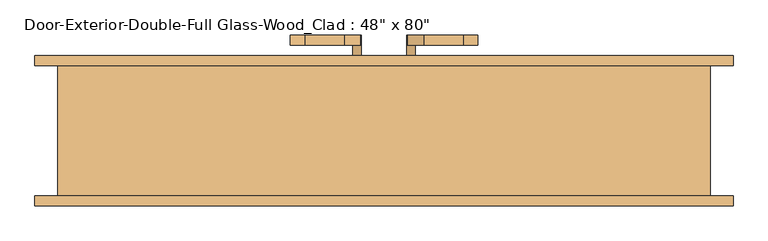
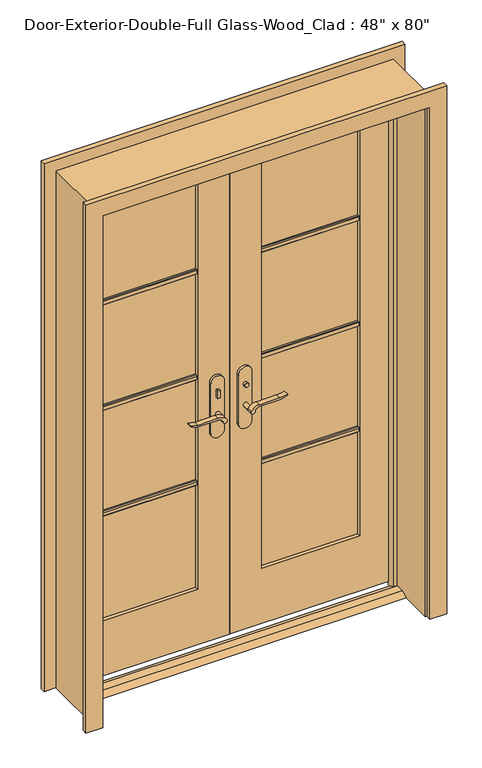
"""IFC4 building model written with IfcOpenShell, lengths in millimetres: door geometry."""

from ifc_helpers import new_model, si_unit, point, frame, frame_2d, origin, place, context, project, spatial, polyline, circle_curve, trimmed, segment, composite_curve, outline, extrude, faceted_brep, source, transform, mapped, element, save


def door_ae07d0c6(model_context):
    return source(origin(), model_context, "Body", "SolidModel", [
        extrude(outline(polyline([(19.05, 12.7), (53.975, 12.7), (79.375, 0.0), (-6.35, 0.0), (19.05, 12.7)])), frame((-609.6, 0.0, 0.0), z_axis=(1.0, 0.0, 0.0), x_axis=(0.0, 1.0, 0.0)), (0.0, 0.0, 1.0), 1219.2),
        extrude(outline(polyline([(-47.4019111, 68.9), (-57.4019111, 68.9), (-57.4019111, 78.9), (-47.4019111, 78.9), (-47.4019111, 68.9)])), frame((0.0, 0.0, 981.9), z_axis=(0.0, 0.0, 1.0), x_axis=(1.0, 0.0, 0.0)), (0.0, 0.0, 1.0), 30.0),
        extrude(outline(composite_curve([segment(trimmed(circle_curve(frame_2d((996.9, -52.4019111)), 8.0), [point((996.9, -60.4019111))], [point((996.9, -44.4019111))], False, "CARTESIAN"), True, "CONTINUOUS"), segment(trimmed(circle_curve(frame_2d((996.9, -52.4019111)), 8.0), [point((996.9, -44.4019111))], [point((996.9, -60.4019111))], False, "CARTESIAN"), True, "CONTINUOUS")], self_intersect=False)), frame((0.0, 133.825, 0.0), z_axis=(0.0, 1.0, 0.0), x_axis=(0.0, 0.0, 1.0)), (0.0, 0.0, 1.0), 10.0),
        extrude(outline(composite_curve([segment(trimmed(circle_curve(frame_2d((897.1555521, -76.0694241)), 37.2832219), [point((919.0523287, -45.8937749))], [point((934.4, -77.7693445))], False, "CARTESIAN"), True, "CONTINUOUS"), segment(polyline([(934.4, -77.7693445), (934.4, -154.045502)]), True, "CONTINUOUS"), segment(trimmed(circle_curve(frame_2d((1017.6850638, -153.9791202)), 83.2850902), [point((934.4, -154.045502))], [point((939.4, -182.4019111))], True, "CARTESIAN"), True, "CONTINUOUS"), segment(polyline([(939.4, -182.4019111), (936.6135558, -182.4019111)]), True, "CONTINUOUS"), segment(trimmed(circle_curve(frame_2d((986.6709207, -150.4622499)), 59.3791355), [point((936.6135558, -182.4019111))], [point((927.4, -154.045502))], False, "CARTESIAN"), True, "CONTINUOUS"), segment(polyline([(927.4, -154.045502), (927.4, -77.7881013)]), True, "CONTINUOUS"), segment(trimmed(circle_curve(frame_2d((909.2738613, -77.7881013)), 18.1261387), [point((927.4, -77.7881013))], [point((914.4, -60.4019111))], True, "CARTESIAN"), True, "CONTINUOUS"), segment(trimmed(circle_curve(frame_2d((914.4, -52.4019111)), 8.0), [point((914.4, -60.4019111))], [point((919.0523287, -45.8937749))], False, "CARTESIAN"), True, "CONTINUOUS")], self_intersect=False)), frame((0.0, 28.9, 0.0), z_axis=(0.0, 1.0, 0.0), x_axis=(0.0, 0.0, 1.0)), (0.0, 0.0, 1.0), 20.0),
        extrude(outline(composite_curve([segment(trimmed(circle_curve(frame_2d((914.4, -52.4019111)), 8.0), [point((914.3999903, -60.4019111))], [point((919.0523287, -45.8937749))], False, "CARTESIAN"), True, "CONTINUOUS"), segment(trimmed(circle_curve(frame_2d((897.1555521, -76.0694241)), 37.2832219), [point((919.0523287, -45.8937749))], [point((934.4, -77.7693445))], False, "CARTESIAN"), True, "CONTINUOUS"), segment(polyline([(934.4, -77.7693445), (934.4, -154.045502)]), True, "CONTINUOUS"), segment(trimmed(circle_curve(frame_2d((1017.6850638, -153.9791202)), 83.2850902), [point((934.4, -154.045502))], [point((939.4, -182.4019111))], True, "CARTESIAN"), True, "CONTINUOUS"), segment(polyline([(939.4, -182.4019111), (936.6135558, -182.4019111)]), True, "CONTINUOUS"), segment(trimmed(circle_curve(frame_2d((986.6709207, -150.4622499)), 59.3791355), [point((936.6135558, -182.4019111))], [point((927.4, -154.045502))], False, "CARTESIAN"), True, "CONTINUOUS"), segment(polyline([(927.4, -154.045502), (927.4, -77.788099)]), True, "CONTINUOUS"), segment(trimmed(circle_curve(frame_2d((909.2738682, -77.788099)), 18.1261318), [point((927.4, -77.788099))], [point((914.3999903, -60.4019111))], True, "CARTESIAN"), True, "CONTINUOUS")], self_intersect=False)), frame((0.0, 163.825, 0.0), z_axis=(0.0, 1.0, 0.0), x_axis=(0.0, 0.0, 1.0)), (0.0, 0.0, 1.0), 20.0),
        extrude(outline(composite_curve([segment(trimmed(circle_curve(frame_2d((914.4, -52.4019111)), 8.0), [point((914.4, -60.4019111))], [point((914.4, -44.4019111))], False, "CARTESIAN"), True, "CONTINUOUS"), segment(trimmed(circle_curve(frame_2d((914.4, -52.4019111)), 8.0), [point((914.4, -44.4019111))], [point((914.4, -60.4019111))], False, "CARTESIAN"), True, "CONTINUOUS")], self_intersect=False)), frame((0.0, 48.9, 0.0), z_axis=(0.0, 1.0, 0.0), x_axis=(0.0, 0.0, 1.0)), (0.0, 0.0, 1.0), 30.0),
        extrude(outline(composite_curve([segment(trimmed(circle_curve(frame_2d((914.4, -52.4019111)), 8.0), [point((914.4, -60.4019111))], [point((914.4, -44.4019111))], False, "CARTESIAN"), True, "CONTINUOUS"), segment(trimmed(circle_curve(frame_2d((914.4, -52.4019111)), 8.0), [point((914.4, -44.4019111))], [point((914.4, -60.4019111))], False, "CARTESIAN"), True, "CONTINUOUS")], self_intersect=False)), frame((0.0, 133.825, 0.0), z_axis=(0.0, 1.0, 0.0), x_axis=(0.0, 0.0, 1.0)), (0.0, 0.0, 1.0), 30.0),
        extrude(outline(composite_curve([segment(polyline([(844.4, -27.4019111), (1039.4, -27.4019111)]), True, "CONTINUOUS"), segment(trimmed(circle_curve(frame_2d((1039.4, -52.4019111)), 25.0), [point((1039.4, -27.4019111))], [point((1039.4, -77.4019111))], False, "CARTESIAN"), True, "CONTINUOUS"), segment(polyline([(1039.4, -77.4019111), (844.4, -77.4019111)]), True, "CONTINUOUS"), segment(trimmed(circle_curve(frame_2d((844.4, -52.4019111)), 25.0), [point((844.4, -77.4019111))], [point((844.4, -27.4019111))], False, "CARTESIAN"), True, "CONTINUOUS")], self_intersect=False)), frame((0.0, 78.9, 0.0), z_axis=(0.0, 1.0, 0.0), x_axis=(0.0, 0.0, 1.0)), (0.0, 0.0, 1.0), 10.0),
        extrude(outline(composite_curve([segment(polyline([(844.4, -27.4019111), (1039.4, -27.4019111)]), True, "CONTINUOUS"), segment(trimmed(circle_curve(frame_2d((1039.4, -52.4019111)), 25.0), [point((1039.4, -27.4019111))], [point((1039.4, -77.4019111))], False, "CARTESIAN"), True, "CONTINUOUS"), segment(polyline([(1039.4, -77.4019111), (844.4, -77.4019111)]), True, "CONTINUOUS"), segment(trimmed(circle_curve(frame_2d((844.4, -52.4019111)), 25.0), [point((844.4, -77.4019111))], [point((844.4, -27.4019111))], False, "CARTESIAN"), True, "CONTINUOUS")], self_intersect=False)), frame((0.0, 123.825, 0.0), z_axis=(0.0, 1.0, 0.0), x_axis=(0.0, 0.0, 1.0)), (0.0, 0.0, 1.0), 10.0),
        extrude(outline(polyline([(47.3875, 143.825), (57.3875, 143.825), (57.3875, 133.825), (47.3875, 133.825), (47.3875, 143.825)])), frame((0.0, 0.0, 981.9), z_axis=(0.0, 0.0, 1.0), x_axis=(1.0, 0.0, 0.0)), (0.0, 0.0, 1.0), 30.0),
        extrude(outline(composite_curve([segment(trimmed(circle_curve(frame_2d((996.9, 52.3875)), 8.0), [point((996.9, 60.3875))], [point((996.9, 44.3875))], False, "CARTESIAN"), True, "CONTINUOUS"), segment(trimmed(circle_curve(frame_2d((996.9, 52.3875)), 8.0), [point((996.9, 44.3875))], [point((996.9, 60.3875))], False, "CARTESIAN"), True, "CONTINUOUS")], self_intersect=False)), frame((0.0, 68.9, 0.0), z_axis=(0.0, 1.0, 0.0), x_axis=(0.0, 0.0, 1.0)), (0.0, 0.0, 1.0), 10.0),
        extrude(outline(composite_curve([segment(trimmed(circle_curve(frame_2d((914.4, 52.3875)), 8.0), [point((919.0523287, 45.8793637))], [point((914.4, 60.3875))], False, "CARTESIAN"), True, "CONTINUOUS"), segment(trimmed(circle_curve(frame_2d((909.2738613, 77.7736901)), 18.1261387), [point((914.4, 60.3875))], [point((927.4, 77.7736901))], True, "CARTESIAN"), True, "CONTINUOUS"), segment(polyline([(927.4, 77.7736901), (927.4, 154.0310909)]), True, "CONTINUOUS"), segment(trimmed(circle_curve(frame_2d((986.6709207, 150.4478388)), 59.3791355), [point((927.4, 154.0310909))], [point((936.6135558, 182.3875))], False, "CARTESIAN"), True, "CONTINUOUS"), segment(polyline([(936.6135558, 182.3875), (939.4, 182.3875)]), True, "CONTINUOUS"), segment(trimmed(circle_curve(frame_2d((1017.6850638, 153.9647091)), 83.2850902), [point((939.4, 182.3875))], [point((934.4, 154.0310909))], True, "CARTESIAN"), True, "CONTINUOUS"), segment(polyline([(934.4, 154.0310909), (934.4, 77.7549333)]), True, "CONTINUOUS"), segment(trimmed(circle_curve(frame_2d((897.1555521, 76.0550129)), 37.2832219), [point((934.4, 77.7549333))], [point((919.0523287, 45.8793637))], False, "CARTESIAN"), True, "CONTINUOUS")], self_intersect=False)), frame((0.0, 163.825, 0.0), z_axis=(0.0, 1.0, 0.0), x_axis=(0.0, 0.0, 1.0)), (0.0, 0.0, 1.0), 20.0),
        extrude(outline(composite_curve([segment(trimmed(circle_curve(frame_2d((909.2738682, 77.7736878)), 18.1261318), [point((914.3999903, 60.3875))], [point((927.4, 77.7736878))], True, "CARTESIAN"), True, "CONTINUOUS"), segment(polyline([(927.4, 77.7736878), (927.4, 154.0310909)]), True, "CONTINUOUS"), segment(trimmed(circle_curve(frame_2d((986.6709207, 150.4478388)), 59.3791355), [point((927.4, 154.0310909))], [point((936.6135558, 182.3875))], False, "CARTESIAN"), True, "CONTINUOUS"), segment(polyline([(936.6135558, 182.3875), (939.4, 182.3875)]), True, "CONTINUOUS"), segment(trimmed(circle_curve(frame_2d((1017.6850638, 153.9647091)), 83.2850902), [point((939.4, 182.3875))], [point((934.4, 154.0310909))], True, "CARTESIAN"), True, "CONTINUOUS"), segment(polyline([(934.4, 154.0310909), (934.4, 77.7549333)]), True, "CONTINUOUS"), segment(trimmed(circle_curve(frame_2d((897.1555521, 76.0550129)), 37.2832219), [point((934.4, 77.7549333))], [point((919.0523287, 45.8793637))], False, "CARTESIAN"), True, "CONTINUOUS"), segment(trimmed(circle_curve(frame_2d((914.4, 52.3875)), 8.0), [point((919.0523287, 45.8793637))], [point((914.3999903, 60.3875))], False, "CARTESIAN"), True, "CONTINUOUS")], self_intersect=False)), frame((0.0, 28.9, 0.0), z_axis=(0.0, 1.0, 0.0), x_axis=(0.0, 0.0, 1.0)), (0.0, 0.0, 1.0), 20.0),
        extrude(outline(composite_curve([segment(trimmed(circle_curve(frame_2d((914.4, 52.3875)), 8.0), [point((914.4, 60.3875))], [point((914.4, 44.3875))], False, "CARTESIAN"), True, "CONTINUOUS"), segment(trimmed(circle_curve(frame_2d((914.4, 52.3875)), 8.0), [point((914.4, 44.3875))], [point((914.4, 60.3875))], False, "CARTESIAN"), True, "CONTINUOUS")], self_intersect=False)), frame((0.0, 133.825, 0.0), z_axis=(0.0, 1.0, 0.0), x_axis=(0.0, 0.0, 1.0)), (0.0, 0.0, 1.0), 30.0),
        extrude(outline(composite_curve([segment(trimmed(circle_curve(frame_2d((914.4, 52.3875)), 8.0), [point((914.4, 60.3875))], [point((914.4, 44.3875))], False, "CARTESIAN"), True, "CONTINUOUS"), segment(trimmed(circle_curve(frame_2d((914.4, 52.3875)), 8.0), [point((914.4, 44.3875))], [point((914.4, 60.3875))], False, "CARTESIAN"), True, "CONTINUOUS")], self_intersect=False)), frame((0.0, 48.9, 0.0), z_axis=(0.0, 1.0, 0.0), x_axis=(0.0, 0.0, 1.0)), (0.0, 0.0, 1.0), 30.0),
        extrude(outline(composite_curve([segment(trimmed(circle_curve(frame_2d((844.4, 52.3875)), 25.0), [point((844.4, 27.3875))], [point((844.4, 77.3875))], False, "CARTESIAN"), True, "CONTINUOUS"), segment(polyline([(844.4, 77.3875), (1039.4, 77.3875)]), True, "CONTINUOUS"), segment(trimmed(circle_curve(frame_2d((1039.4, 52.3875)), 25.0), [point((1039.4, 77.3875))], [point((1039.4, 27.3875))], False, "CARTESIAN"), True, "CONTINUOUS"), segment(polyline([(1039.4, 27.3875), (844.4, 27.3875)]), True, "CONTINUOUS")], self_intersect=False)), frame((0.0, 123.825, 0.0), z_axis=(0.0, 1.0, 0.0), x_axis=(0.0, 0.0, 1.0)), (0.0, 0.0, 1.0), 10.0),
        extrude(outline(composite_curve([segment(trimmed(circle_curve(frame_2d((844.4, 52.3875)), 25.0), [point((844.4, 27.3875))], [point((844.4, 77.3875))], False, "CARTESIAN"), True, "CONTINUOUS"), segment(polyline([(844.4, 77.3875), (1039.4, 77.3875)]), True, "CONTINUOUS"), segment(trimmed(circle_curve(frame_2d((1039.4, 52.3875)), 25.0), [point((1039.4, 77.3875))], [point((1039.4, 27.3875))], False, "CARTESIAN"), True, "CONTINUOUS"), segment(polyline([(1039.4, 27.3875), (844.4, 27.3875)]), True, "CONTINUOUS")], self_intersect=False)), frame((0.0, 78.9, 0.0), z_axis=(0.0, 1.0, 0.0), x_axis=(0.0, 0.0, 1.0)), (0.0, 0.0, 1.0), 10.0),
        extrude(outline(polyline([(102.87, 1502.171875), (102.87, 1483.121875), (96.52, 1483.121875), (93.345, 1486.296875), (93.345, 1498.996875), (96.52, 1502.171875), (102.87, 1502.171875)])), frame((120.65, 0.0, 0.0), z_axis=(1.0, 0.0, 0.0), x_axis=(0.0, 1.0, 0.0)), (0.0, 0.0, 1.0), 368.3),
        extrude(outline(polyline([(102.87, 1081.88125), (102.87, 1062.83125), (96.52, 1062.83125), (93.345, 1066.00625), (93.345, 1078.70625), (96.52, 1081.88125), (102.87, 1081.88125)])), frame((120.65, 0.0, 0.0), z_axis=(1.0, 0.0, 0.0), x_axis=(0.0, 1.0, 0.0)), (0.0, 0.0, 1.0), 368.3),
        extrude(outline(polyline([(102.87, 661.590625), (102.87, 642.540625), (96.52, 642.540625), (93.345, 645.715625), (93.345, 658.415625), (96.52, 661.590625), (102.87, 661.590625)])), frame((120.65, 0.0, 0.0), z_axis=(1.0, 0.0, 0.0), x_axis=(0.0, 1.0, 0.0)), (0.0, 0.0, 1.0), 368.3),
        extrude(outline(polyline([(109.855, 1502.171875), (116.205, 1502.171875), (119.38, 1498.996875), (119.38, 1486.296875), (116.205, 1483.121875), (109.855, 1483.121875), (109.855, 1502.171875)])), frame((-488.95, 0.0, 0.0), z_axis=(1.0, 0.0, 0.0), x_axis=(0.0, 1.0, 0.0)), (0.0, 0.0, 1.0), 368.3),
        extrude(outline(polyline([(109.855, 1081.88125), (116.205, 1081.88125), (119.38, 1078.70625), (119.38, 1066.00625), (116.205, 1062.83125), (109.855, 1062.83125), (109.855, 1081.88125)])), frame((-488.95, 0.0, 0.0), z_axis=(1.0, 0.0, 0.0), x_axis=(0.0, 1.0, 0.0)), (0.0, 0.0, 1.0), 368.3),
        extrude(outline(polyline([(109.855, 661.590625), (116.205, 661.590625), (119.38, 658.415625), (119.38, 645.715625), (116.205, 642.540625), (109.855, 642.540625), (109.855, 661.590625)])), frame((-488.95, 0.0, 0.0), z_axis=(1.0, 0.0, 0.0), x_axis=(0.0, 1.0, 0.0)), (0.0, 0.0, 1.0), 368.3),
        extrude(outline(polyline([(109.855, 1502.171875), (116.205, 1502.171875), (119.38, 1498.996875), (119.38, 1486.296875), (116.205, 1483.121875), (109.855, 1483.121875), (109.855, 1502.171875)])), frame((120.65, 0.0, 0.0), z_axis=(1.0, 0.0, 0.0), x_axis=(0.0, 1.0, 0.0)), (0.0, 0.0, 1.0), 368.3),
        extrude(outline(polyline([(109.855, 1081.88125), (116.205, 1081.88125), (119.38, 1078.70625), (119.38, 1066.00625), (116.205, 1062.83125), (109.855, 1062.83125), (109.855, 1081.88125)])), frame((120.65, 0.0, 0.0), z_axis=(1.0, 0.0, 0.0), x_axis=(0.0, 1.0, 0.0)), (0.0, 0.0, 1.0), 368.3),
        extrude(outline(polyline([(109.855, 661.590625), (116.205, 661.590625), (119.38, 658.415625), (119.38, 645.715625), (116.205, 642.540625), (109.855, 642.540625), (109.855, 661.590625)])), frame((120.65, 0.0, 0.0), z_axis=(1.0, 0.0, 0.0), x_axis=(0.0, 1.0, 0.0)), (0.0, 0.0, 1.0), 368.3),
        extrude(outline(polyline([(102.87, 1502.171875), (102.87, 1483.121875), (96.52, 1483.121875), (93.345, 1486.296875), (93.345, 1498.996875), (96.52, 1502.171875), (102.87, 1502.171875)])), frame((-488.95, 0.0, 0.0), z_axis=(1.0, 0.0, 0.0), x_axis=(0.0, 1.0, 0.0)), (0.0, 0.0, 1.0), 368.3),
        extrude(outline(polyline([(102.87, 1081.88125), (102.87, 1062.83125), (96.52, 1062.83125), (93.345, 1066.00625), (93.345, 1078.70625), (96.52, 1081.88125), (102.87, 1081.88125)])), frame((-488.95, 0.0, 0.0), z_axis=(1.0, 0.0, 0.0), x_axis=(0.0, 1.0, 0.0)), (0.0, 0.0, 1.0), 368.3),
        extrude(outline(polyline([(102.87, 661.590625), (102.87, 642.540625), (96.52, 642.540625), (93.345, 645.715625), (93.345, 658.415625), (96.52, 661.590625), (102.87, 661.590625)])), frame((-488.95, 0.0, 0.0), z_axis=(1.0, 0.0, 0.0), x_axis=(0.0, 1.0, 0.0)), (0.0, 0.0, 1.0), 368.3),
        extrude(outline(polyline([(0.0, 615.95), (0.0, 679.45), (2101.85, 679.45), (2101.85, -679.45), (0.0, -679.45), (0.0, -615.95), (2038.35, -615.95), (2038.35, 615.95), (0.0, 615.95)])), frame((0.0, -149.225, 0.0), z_axis=(0.0, 1.0, 0.0), x_axis=(0.0, 0.0, 1.0)), (0.0, 0.0, 1.0), 19.05),
        extrude(outline(polyline([(0.0, 615.95), (0.0, 679.45), (2101.85, 679.45), (2101.85, -679.45), (0.0, -679.45), (0.0, -615.95), (2038.35, -615.95), (2038.35, 615.95), (0.0, 615.95)])), frame((0.0, 123.825, 0.0), z_axis=(0.0, 1.0, 0.0), x_axis=(0.0, 0.0, 1.0)), (0.0, 0.0, 1.0), 19.05),
        faceted_brep([(635.0, 123.825, 0.0), (635.0, -130.175, 0.0), (609.6, -130.175, 0.0), (609.6, 53.975, 0.0), (596.9, 53.975, 0.0), (596.9, 88.9, 0.0), (609.6, 88.9, 0.0), (609.6, 123.825, 0.0), (635.0, 123.825, 2057.4), (635.0, -130.175, 2057.4), (-635.0, -130.175, 2057.4), (-635.0, -130.175, 0.0), (-609.6, -130.175, 0.0), (-609.6, -130.175, 2032.0), (609.6, -130.175, 2032.0), (609.6, 53.975, 2032.0), (-609.6, 53.975, 2032.0), (-609.6, 53.975, 0.0), (-596.9, 53.975, 0.0), (-596.9, 53.975, 2019.3), (596.9, 53.975, 2019.3), (596.9, 88.9, 2019.3), (1.5875, 88.9, 2019.3), (-1.6019111, 88.9, 2019.3), (-596.9, 88.9, 2019.3), (-596.9, 88.9, 0.0), (-609.6, 88.9, 0.0), (-609.6, 88.9, 2032.0), (-1.6019111, 88.9, 2032.0), (1.5875, 88.9, 2032.0), (609.6, 88.9, 2032.0), (609.6, 123.825, 2032.0), (1.5875, 123.825, 2032.0), (-1.6019111, 123.825, 2032.0), (-609.6, 123.825, 2032.0), (-609.6, 123.825, 0.0), (-635.0, 123.825, 0.0), (-635.0, 123.825, 2057.4)], [[[0, 1, 2, 3, 4, 5, 6, 7]], [[1, 0, 8, 9]], [[2, 1, 9, 10, 11, 12, 13, 14]], [[3, 2, 14, 15]], [[4, 3, 15, 16, 17, 18, 19, 20]], [[5, 4, 20, 21]], [[6, 5, 21, 22, 23, 24, 25, 26, 27, 28, 29, 30]], [[7, 6, 30, 31]], [[0, 7, 31, 32, 33, 34, 35, 36, 37, 8]], [[9, 8, 37, 10]], [[14, 13, 16, 15]], [[20, 19, 24, 23, 22, 21]], [[31, 30, 29, 28, 27, 34, 33, 32]], [[12, 11, 36, 35, 26, 25, 18, 17]], [[11, 10, 37, 36]], [[13, 12, 17, 16]], [[19, 18, 25, 24]], [[27, 26, 35, 34]]]),
        extrude(outline(polyline([(12.7, 609.6), (2032.0, 609.6), (2032.0, 1.5875), (12.7, 1.5875), (12.7, 609.6)]), holes=[polyline([(1912.9375, 120.65), (1912.9375, 488.95), (231.775, 488.95), (231.775, 120.65), (1912.9375, 120.65)])]), frame((0.0, 88.9, 0.0), z_axis=(0.0, 1.0, 0.0), x_axis=(0.0, 0.0, 1.0)), (0.0, 0.0, 1.0), 34.925),
        extrude(outline(polyline([(2032.0, -609.6), (12.7, -609.6), (12.7, -1.6019111), (2032.0, -1.6019111), (2032.0, -609.6)]), holes=[polyline([(231.775, -488.95), (1912.9375, -488.95), (1912.9375, -120.65), (231.775, -120.65), (231.775, -488.95)])]), frame((0.0, 88.9, 0.0), z_axis=(0.0, 1.0, 0.0), x_axis=(0.0, 0.0, 1.0)), (0.0, 0.0, 1.0), 34.925),
        extrude(outline(polyline([(488.95, 102.87), (120.65, 102.87), (120.65, 109.855), (488.95, 109.855), (488.95, 102.87)])), frame((0.0, 0.0, 231.775), z_axis=(0.0, 0.0, 1.0), x_axis=(1.0, 0.0, 0.0)), (0.0, 0.0, 1.0), 1681.1625),
        extrude(outline(polyline([(-120.65, 102.87), (-488.95, 102.87), (-488.95, 109.855), (-120.65, 109.855), (-120.65, 102.87)])), frame((0.0, 0.0, 231.775), z_axis=(0.0, 0.0, 1.0), x_axis=(1.0, 0.0, 0.0)), (0.0, 0.0, 1.0), 1681.1625),
    ])


if __name__ == "__main__":
    model = new_model("IFC4")
    model_context = context("Model", 3, world=origin())
    ifc_project = project(units=[si_unit("LENGTHUNIT", "METRE", prefix="MILLI")], contexts=[model_context])
    site = spatial("IfcSite", under=ifc_project)
    building = spatial("IfcBuilding", under=site)
    placement = place(None, origin())
    door_shape = door_ae07d0c6(model_context)
    element("IfcDoor", 1, ObjectType="Door-Exterior-Double-Full Glass-Wood_Clad : 48\" x 80\"", at=placement, inside=building, context=model_context, shape_type="MappedRepresentation", body=[
        mapped(door_shape, transform((0.0, 0.0, 0.0), x_axis=(1.0, 0.0, 0.0), y_axis=(0.0, 1.0, 0.0), z_axis=(0.0, 0.0, 1.0))),
    ])
    save(model, "model.ifc")

# Revit data of these elements
# Type "Door-Exterior-Double-Full Glass-Wood_Clad : 48\" x 80\""
#   Type Mark = "16"
#   Assembly Code = "B2030100"
#   Analytic Construction = "French door, wood frame with double glass"
#   Top Rail = 0' - 4 11/16"
#   Threshold Offset [instance default] = 0' - 0 1/2"
#   Thickness = 0' - 1 3/8"
#   Thermal Resistance (R) = 1.9158 (h·ft²·°F)/BTU
#   Swing Angle [instance default] = 90.00°
#   Stiles = 0' - 4 3/4"
#   Rough Width = 4' - 2"
#   Rough Height = 6' - 9"
#   Panel Width = 2' - 0"
#   Door Offset [instance default] = 0' - 0"
#   Height = 6' - 8"
#   Width = 4' - 0"
#   Heat Transfer Coefficient (U) = 0.5220 BTU/(h·ft²·°F)
#   Bottom Rail = 0' - 9 1/8"
#   Exterior Trim [instance default] = yes
#   Threshold [instance default] = yes
#   Show Grill [instance default] = yes
#   Function = 1
#   Trim Material = Cherry
#   Threshold Material = Cherry
#   Panel Material = Cherry
#   Glazing = Glass
#   Frame Material = Cherry
#   Door Handle Material = Aluminum
#   Visual Light Transmittance = 0
#   Solar Heat Gain Coefficient = 0
#   Wall Closure = (empty or 0)
#   Construction Type = (empty or 0)
# Element 1 (IfcDoor, "Door-Exterior-Double-Full Glass-Wood_Clad : 48\" x 80\"")
#   Materials on its faces: "Cherry", "Aluminum", "Glass"
# Materials
#   "Cherry": class "Wood", colour RGB 226 177 128, transparency 0, Description = "Prunus Serotina", Cost = 0
#   "Glass": class "Glass", colour RGB 0 128 192, transparency 0.75, Description = "Soda Lime Glass", Cost = 0
#   "Aluminum": class "Metal", colour RGB 247 247 247, transparency 0, Description = "Aluminum 6061", Cost = 0
